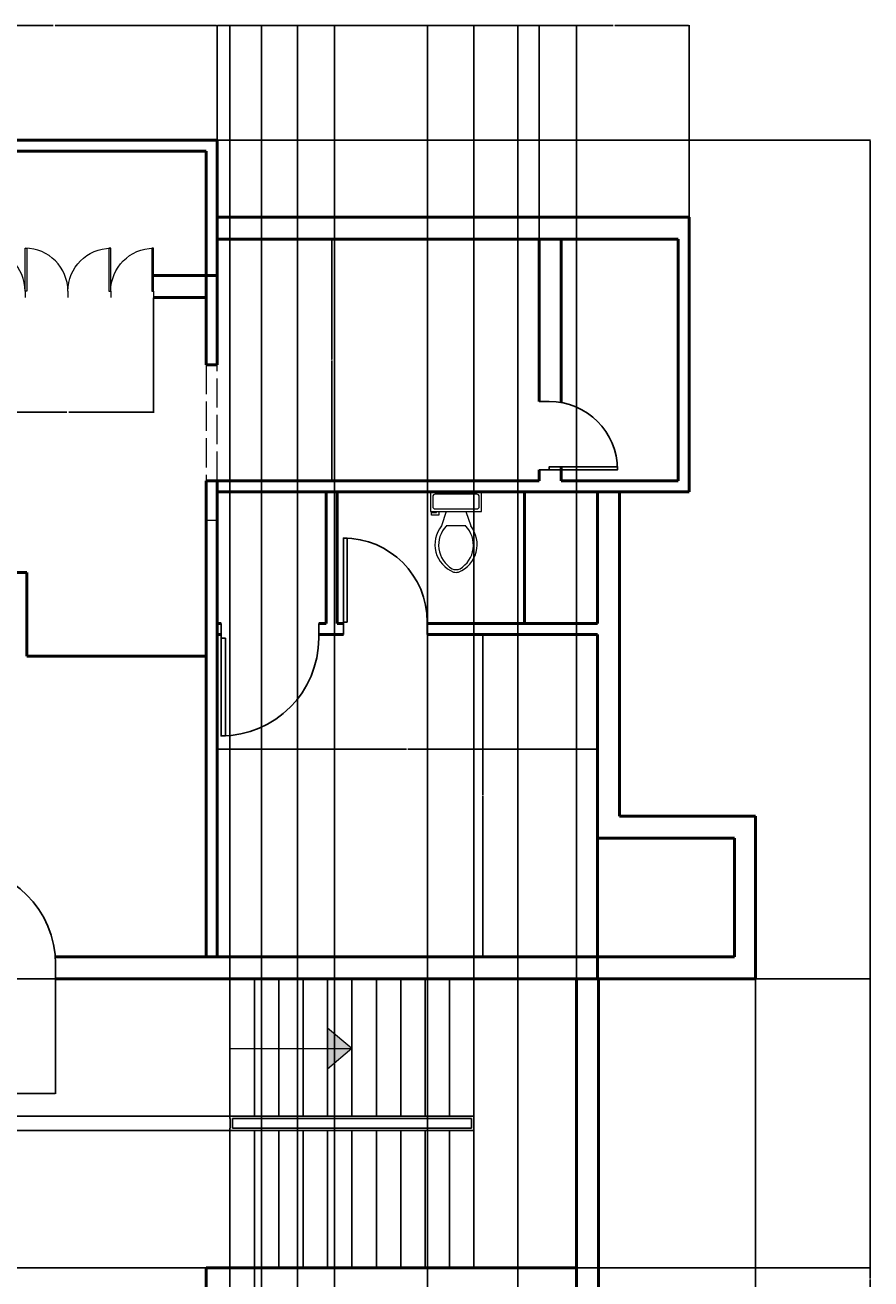
# Model space of a CAD drawing. Units: inches. Extents: x 2032 to 3981, y 840 to 2177.
# Tile 5 of 6: x 2378 to 2725, y 1354 to 1868. Entities that reach past the tile are written whole.
import ezdxf

# ---------------------------------------------------------------- set-up
doc = ezdxf.new("R2010")
doc.units = ezdxf.units.IN
doc.linetypes.add('ACAD_ISO02W100', pattern=[15, 12, -3])
for name, color, linetype, lineweight in [('A-ANNO-DIMS', 2, 'Continuous', 18), ('A-ANNO-SYMB', 2, 'Continuous', 18), ('A-DOOR', 3, 'Continuous', 25), ('A-FLOR-FIXT', 9, 'Continuous', 18), ('A-FLOR-STRS', 7, 'Continuous', 25), ('A-GLAZ', 4, 'Continuous', 18), ('A-WALL', 7, 'Continuous', 50), ('A-WALL-OVHD', 8, 'ACAD_ISO02W100', 18)]:
    doc.layers.add(name, color=color, linetype=linetype, lineweight=lineweight)
doc.styles.get("Standard").update_dxf_attribs({"font": 'arial.ttf'})
doc.dimstyles.get("Standard").update_dxf_attribs({"dimtxt": 0.18, "dimasz": 0.18, "dimexe": 0.18, "dimexo": 0.0625, "dimgap": 0.09, "dimtad": 0, "dimtih": 1, "dimtoh": 1, "dimdec": 4, "dimzin": 0, "dimdsep": 46, "dimtxsty": 'Standard', "dimcen": 0.09, "dimadec": 0, "dimazin": 0, "dimtfac": 1, "dimtdec": 4, "dimtofl": 0, "dimtmove": 0, "dimatfit": 3, "dimfxl": 1, "dimtolj": 1, "dimtzin": 0, "dimarcsym": 0})

# ---------------------------------------------------------------- blocks, each defined once
blk = doc.blocks.new('*U2')
for p, q in [((0, 0), (0, -6)), ((40, 0), (40, -6))]:
    blk.add_line(p, q)
blk.add_lwpolyline([(0, 0), (0, 40), (1.75, 40), (1.75, 0)], close=True)
blk.add_arc((0, 0), 40, 0, 90)
blk = doc.blocks.new('*U4')
for p, q in [((9.5, -6), (9.5, -2)), ((-10, -8.5), (-8, -8.5)), ((-10, -9.5), (-10, -8.5)), ((-7, -9.5), (-10, -9.5)), ((-8, -8.5), (-8, -8)), ((-7, -8), (-7, -9.5)), ((-4, -8), (-6, -14)), ((4, -8), (6, -14)), ((4, -14), (-4, -14))]:
    blk.add_line(p, q)
blk.add_lwpolyline([(10.5, -8), (10.5, 0), (-10.5, 0), (-10.5, -8)], close=True)
for points in [[(-9.5, -2), (-9.5, -6)], [(8.5, -1), (-8.5, -1)], [(-8.5, -7), (8.5, -7)]]:
    blk.add_lwpolyline(points)
for centre, radius, start, end in [((-8.62, -1.88), 0.884, 81.8699, 188.1301), ((8.62, -1.88), 0.884, 351.8699, 98.1301), ((-8.62, -6.12), 0.884, 171.8699, 278.1301), ((8.62, -6.12), 0.884, 261.8699, 8.1301), ((3.52, -21.58), 12.17, 141.4691, 247.9714), ((4.2, -21.82), 11.33, 136.3677, 238.9468), ((-3.52, -21.58), 12.17, 292.0284, 38.5307), ((-4.2, -21.82), 11.33, 301.053, 43.6321), ((0, -27.88), 4, 245.7318, 294.2682), ((0, -29), 4, 254.8605, 285.1395)]:
    blk.add_arc(centre, radius, start, end)
blk = doc.blocks.new('*D14')
at = {"layer": 'A-ANNO-DIMS', "color": 0, "lineweight": -2, "transparency": 16777216}
for p, q in [((2078.89, 1518.9), (2078.89, 840.08)), ((2677.35, 1476.9), (2677.35, 840.08)), ((2079.07, 840.26), (2377.73, 840.26)), ((2677.17, 840.26), (2378.52, 840.26))]:
    blk.add_line(p, q, dxfattribs=at)
at = {"layer": 'A-ANNO-DIMS', "color": 0, "lineweight": 100, "transparency": 16777216}
for points in [[(2079.07, 840.29), (2079.07, 840.23), (2078.89, 840.26)], [(2677.17, 840.29), (2677.17, 840.23), (2677.35, 840.26)]]:
    blk.add_solid(points, dxfattribs=at)
at = {"layer": 'Defpoints', "color": 0, "lineweight": 100, "transparency": 16777216}
for p in [(2078.89, 1518.96), (2677.35, 1476.96), (2677.35, 840.26)]:
    blk.add_point(p, dxfattribs=at)
at = {"layer": 'A-ANNO-DIMS', "color": 0, "transparency": 16777216, "insert": (2378.12, 840.26), "char_height": 0.18, "attachment_point": 5}
blk.add_mtext('\\A1;598.5', dxfattribs=at)
blk = doc.blocks.new('*D15')
at = {"layer": 'A-ANNO-DIMS', "color": 0, "lineweight": -2, "transparency": 16777216}
for p, q in [((2456.69, 1820.52), (2724.53, 1820.52)), ((2724.35, 1820.34), (2724.35, 1354.07)), ((2724.35, 887.44), (2724.35, 1353.71)), ((2476.27, 887.26), (2724.53, 887.26))]:
    blk.add_line(p, q, dxfattribs=at)
at = {"layer": 'A-ANNO-DIMS', "color": 0, "lineweight": 100, "transparency": 16777216}
for points in [[(2724.32, 1820.34), (2724.38, 1820.34), (2724.35, 1820.52)], [(2724.32, 887.44), (2724.38, 887.44), (2724.35, 887.26)]]:
    blk.add_solid(points, dxfattribs=at)
at = {"layer": 'Defpoints', "color": 0, "lineweight": 100, "transparency": 16777216}
for p in [(2456.63, 1820.52), (2476.21, 887.26), (2724.35, 887.26)]:
    blk.add_point(p, dxfattribs=at)
at = {"layer": 'A-ANNO-DIMS', "color": 0, "transparency": 16777216, "insert": (2724.35, 1353.89), "char_height": 0.18, "attachment_point": 5}
blk.add_mtext('\\A1;933.3', dxfattribs=at)
blk = doc.blocks.new('*D19')
at = {"layer": 'A-ANNO-DIMS', "color": 0, "lineweight": -2, "transparency": 16777216}
for p, q in [((2323.13, 1820.58), (2323.13, 1867.7)), ((2323.31, 1867.52), (2389.49, 1867.52)), ((2456.45, 1867.52), (2390.26, 1867.52)), ((2456.63, 1820.58), (2456.63, 1867.7))]:
    blk.add_line(p, q, dxfattribs=at)
at = {"layer": 'A-ANNO-DIMS', "color": 0, "lineweight": 100, "transparency": 16777216}
for points in [[(2323.31, 1867.55), (2323.31, 1867.49), (2323.13, 1867.52)], [(2456.45, 1867.55), (2456.45, 1867.49), (2456.63, 1867.52)]]:
    blk.add_solid(points, dxfattribs=at)
at = {"layer": 'Defpoints', "color": 0, "lineweight": 100, "transparency": 16777216}
for p in [(2456.63, 1867.52), (2323.13, 1820.52), (2456.63, 1820.52)]:
    blk.add_point(p, dxfattribs=at)
at = {"layer": 'A-ANNO-DIMS', "color": 0, "transparency": 16777216, "insert": (2389.88, 1867.52), "char_height": 0.18, "attachment_point": 5}
blk.add_mtext('\\A1;133.5', dxfattribs=at)
blk = doc.blocks.new('*D20')
at = {"layer": 'A-ANNO-DIMS', "color": 0, "lineweight": -2, "transparency": 16777216}
for p, q in [((2456.63, 1820.58), (2456.63, 1867.7)), ((2456.81, 1867.52), (2522.35, 1867.52)), ((2588.45, 1867.52), (2522.91, 1867.52)), ((2588.63, 1780.02), (2588.63, 1867.7))]:
    blk.add_line(p, q, dxfattribs=at)
at = {"layer": 'A-ANNO-DIMS', "color": 0, "lineweight": 100, "transparency": 16777216}
for points in [[(2456.81, 1867.55), (2456.81, 1867.49), (2456.63, 1867.52)], [(2588.45, 1867.55), (2588.45, 1867.49), (2588.63, 1867.52)]]:
    blk.add_solid(points, dxfattribs=at)
at = {"layer": 'Defpoints', "color": 0, "lineweight": 100, "transparency": 16777216}
for p in [(2588.63, 1867.52), (2456.63, 1820.52), (2588.63, 1779.96)]:
    blk.add_point(p, dxfattribs=at)
at = {"layer": 'A-ANNO-DIMS', "color": 0, "transparency": 16777216, "insert": (2522.63, 1867.52), "char_height": 0.18, "attachment_point": 5}
blk.add_mtext('\\A1;132', dxfattribs=at)
blk = doc.blocks.new('*D21')
at = {"layer": 'A-ANNO-DIMS', "color": 0, "lineweight": -2, "transparency": 16777216}
for p, q in [((2588.63, 1780.02), (2588.63, 1867.7)), ((2588.81, 1867.52), (2619.05, 1867.52)), ((2649.95, 1867.52), (2619.7, 1867.52)), ((2650.13, 1789.02), (2650.13, 1867.7))]:
    blk.add_line(p, q, dxfattribs=at)
at = {"layer": 'A-ANNO-DIMS', "color": 0, "lineweight": 100, "transparency": 16777216}
for points in [[(2588.81, 1867.55), (2588.81, 1867.49), (2588.63, 1867.52)], [(2649.95, 1867.55), (2649.95, 1867.49), (2650.13, 1867.52)]]:
    blk.add_solid(points, dxfattribs=at)
at = {"layer": 'Defpoints', "color": 0, "lineweight": 100, "transparency": 16777216}
for p in [(2650.13, 1867.52), (2650.13, 1788.96), (2588.63, 1779.96)]:
    blk.add_point(p, dxfattribs=at)
at = {"layer": 'A-ANNO-DIMS', "color": 0, "transparency": 16777216, "insert": (2619.38, 1867.52), "char_height": 0.18, "attachment_point": 5}
blk.add_mtext('\\A1;61.5', dxfattribs=at)
blk = doc.blocks.new('*D31')
at = {"layer": 'A-ANNO-DIMS', "color": 0, "lineweight": -2, "transparency": 16777216}
for p, q in [((2456.69, 1779.96), (2503.81, 1779.96)), ((2503.63, 1779.78), (2503.63, 1730.64)), ((2503.63, 1681.14), (2503.63, 1730.28)), ((2456.69, 1680.96), (2503.81, 1680.96))]:
    blk.add_line(p, q, dxfattribs=at)
at = {"layer": 'A-ANNO-DIMS', "color": 0, "lineweight": 100, "transparency": 16777216}
for points in [[(2503.6, 1779.78), (2503.66, 1779.78), (2503.63, 1779.96)], [(2503.6, 1681.14), (2503.66, 1681.14), (2503.63, 1680.96)]]:
    blk.add_solid(points, dxfattribs=at)
at = {"layer": 'Defpoints', "color": 0, "lineweight": 100, "transparency": 16777216}
for p in [(2456.63, 1779.96), (2456.63, 1680.96), (2503.63, 1680.96)]:
    blk.add_point(p, dxfattribs=at)
at = {"layer": 'A-ANNO-DIMS', "color": 0, "transparency": 16777216, "insert": (2503.63, 1730.46), "char_height": 0.18, "attachment_point": 5}
blk.add_mtext('\\A1;99', dxfattribs=at)
blk = doc.blocks.new('*D32')
at = {"layer": 'A-ANNO-DIMS', "color": 0, "lineweight": -2, "transparency": 16777216}
for p, q in [((2360.39, 1756), (2360.39, 1708.89)), ((2430.64, 1756), (2430.64, 1708.89)), ((2360.57, 1709.07), (2395.12, 1709.07)), ((2430.46, 1709.07), (2395.91, 1709.07))]:
    blk.add_line(p, q, dxfattribs=at)
at = {"layer": 'A-ANNO-DIMS', "color": 0, "lineweight": 100, "transparency": 16777216}
for points in [[(2360.57, 1709.1), (2360.57, 1709.04), (2360.39, 1709.07)], [(2430.46, 1709.1), (2430.46, 1709.04), (2430.64, 1709.07)]]:
    blk.add_solid(points, dxfattribs=at)
at = {"layer": 'Defpoints', "color": 0, "lineweight": 100, "transparency": 16777216}
for p in [(2360.39, 1756.07), (2430.64, 1756.07), (2360.39, 1709.07)]:
    blk.add_point(p, dxfattribs=at)
at = {"layer": 'A-ANNO-DIMS', "color": 0, "transparency": 16777216, "insert": (2395.51, 1709.07), "char_height": 0.18, "attachment_point": 5}
blk.add_mtext('\\A1;70.24', dxfattribs=at)
blk = doc.blocks.new('*D35')
at = {"layer": 'A-ANNO-DIMS', "color": 0, "lineweight": -2, "transparency": 16777216}
for p, q in [((2456.63, 1617.9), (2456.63, 1570.78)), ((2612.63, 1617.9), (2612.63, 1570.78)), ((2456.81, 1570.96), (2534.35, 1570.96)), ((2612.45, 1570.96), (2534.91, 1570.96))]:
    blk.add_line(p, q, dxfattribs=at)
at = {"layer": 'A-ANNO-DIMS', "color": 0, "lineweight": 100, "transparency": 16777216}
for points in [[(2456.81, 1570.99), (2456.81, 1570.93), (2456.63, 1570.96)], [(2612.45, 1570.99), (2612.45, 1570.93), (2612.63, 1570.96)]]:
    blk.add_solid(points, dxfattribs=at)
at = {"layer": 'Defpoints', "color": 0, "lineweight": 100, "transparency": 16777216}
for p in [(2456.63, 1617.96), (2612.63, 1617.96), (2456.63, 1570.96)]:
    blk.add_point(p, dxfattribs=at)
at = {"layer": 'A-ANNO-DIMS', "color": 0, "transparency": 16777216, "insert": (2534.63, 1570.96), "char_height": 0.18, "attachment_point": 5}
blk.add_mtext('\\A1;156', dxfattribs=at)
blk = doc.blocks.new('*D36')
at = {"layer": 'A-ANNO-DIMS', "color": 0, "lineweight": -2, "transparency": 16777216}
for p, q in [((2612.57, 1617.96), (2565.45, 1617.96)), ((2565.63, 1617.78), (2565.63, 1552.14)), ((2565.63, 1486.14), (2565.63, 1551.78)), ((2612.57, 1485.96), (2565.45, 1485.96))]:
    blk.add_line(p, q, dxfattribs=at)
at = {"layer": 'A-ANNO-DIMS', "color": 0, "lineweight": 100, "transparency": 16777216}
for points in [[(2565.6, 1617.78), (2565.66, 1617.78), (2565.63, 1617.96)], [(2565.6, 1486.14), (2565.66, 1486.14), (2565.63, 1485.96)]]:
    blk.add_solid(points, dxfattribs=at)
at = {"layer": 'Defpoints', "color": 0, "lineweight": 100, "transparency": 16777216}
for p in [(2565.63, 1617.96), (2612.63, 1617.96), (2612.63, 1485.96)]:
    blk.add_point(p, dxfattribs=at)
at = {"layer": 'A-ANNO-DIMS', "color": 0, "transparency": 16777216, "insert": (2565.63, 1551.96), "char_height": 0.18, "attachment_point": 5}
blk.add_mtext('\\A1;132', dxfattribs=at)
blk = doc.blocks.new('*D37')
at = {"layer": 'A-ANNO-DIMS', "color": 0, "lineweight": -2, "transparency": 16777216}
for p, q in [((2350.44, 1476.9), (2350.44, 1429.78)), ((2390.44, 1476.9), (2390.44, 1429.78)), ((2350.62, 1429.96), (2370.22, 1429.96)), ((2390.26, 1429.96), (2370.66, 1429.96))]:
    blk.add_line(p, q, dxfattribs=at)
at = {"layer": 'A-ANNO-DIMS', "color": 0, "lineweight": 100, "transparency": 16777216}
for points in [[(2350.62, 1429.99), (2350.62, 1429.93), (2350.44, 1429.96)], [(2390.26, 1429.99), (2390.26, 1429.93), (2390.44, 1429.96)]]:
    blk.add_solid(points, dxfattribs=at)
at = {"layer": 'Defpoints', "color": 0, "lineweight": 100, "transparency": 16777216}
for p in [(2350.44, 1476.96), (2390.44, 1476.96), (2350.44, 1429.96)]:
    blk.add_point(p, dxfattribs=at)
at = {"layer": 'A-ANNO-DIMS', "color": 0, "transparency": 16777216, "insert": (2370.44, 1429.96), "char_height": 0.18, "attachment_point": 5}
blk.add_mtext('\\A1;40', dxfattribs=at)
blk = doc.blocks.new('*D51')
at = {"layer": 'A-ANNO-DIMS', "color": 0, "lineweight": -2, "transparency": 16777216}
for p, q in [((2474.93, 1231.02), (2474.93, 1867.7)), ((2475.11, 1867.52), (2481.81, 1867.52)), ((2489.42, 1867.52), (2482.72, 1867.52)), ((2489.6, 1231.02), (2489.6, 1867.7))]:
    blk.add_line(p, q, dxfattribs=at)
at = {"layer": 'A-ANNO-DIMS', "color": 0, "lineweight": 100, "transparency": 16777216}
for points in [[(2475.11, 1867.55), (2475.11, 1867.49), (2474.93, 1867.52)], [(2489.42, 1867.55), (2489.42, 1867.49), (2489.6, 1867.52)]]:
    blk.add_solid(points, dxfattribs=at)
at = {"layer": 'Defpoints', "color": 0, "lineweight": 100, "transparency": 16777216}
for p in [(2489.6, 1867.52), (2474.93, 1230.96), (2489.6, 1230.96)]:
    blk.add_point(p, dxfattribs=at)
at = {"layer": 'A-ANNO-DIMS', "color": 0, "transparency": 16777216, "insert": (2482.27, 1867.52), "char_height": 0.18, "attachment_point": 5}
blk.add_mtext('\\A1;14.668', dxfattribs=at)
blk = doc.blocks.new('*D52')
at = {"layer": 'A-ANNO-DIMS', "color": 0, "lineweight": -2, "transparency": 16777216}
for p, q in [((2489.6, 1231.02), (2489.6, 1867.7)), ((2489.78, 1867.52), (2496.71, 1867.52)), ((2504.55, 1867.52), (2497.62, 1867.52)), ((2504.73, 1228.5), (2504.73, 1867.7))]:
    blk.add_line(p, q, dxfattribs=at)
at = {"layer": 'A-ANNO-DIMS', "color": 0, "lineweight": 100, "transparency": 16777216}
for points in [[(2489.78, 1867.55), (2489.78, 1867.49), (2489.6, 1867.52)], [(2504.55, 1867.55), (2504.55, 1867.49), (2504.73, 1867.52)]]:
    blk.add_solid(points, dxfattribs=at)
at = {"layer": 'Defpoints', "color": 0, "lineweight": 100, "transparency": 16777216}
for p in [(2504.73, 1867.52), (2489.6, 1230.96), (2504.73, 1228.44)]:
    blk.add_point(p, dxfattribs=at)
at = {"layer": 'A-ANNO-DIMS', "color": 0, "transparency": 16777216, "insert": (2497.17, 1867.52), "char_height": 0.18, "attachment_point": 5}
blk.add_mtext('\\A1;15.127', dxfattribs=at)
blk = doc.blocks.new('*D53')
at = {"layer": 'A-ANNO-DIMS', "color": 0, "lineweight": -2, "transparency": 16777216}
for p, q in [((2504.73, 1228.5), (2504.73, 1867.7)), ((2504.91, 1867.52), (2523.42, 1867.52)), ((2542.71, 1867.52), (2524.2, 1867.52)), ((2542.89, 1228.5), (2542.89, 1867.7))]:
    blk.add_line(p, q, dxfattribs=at)
at = {"layer": 'A-ANNO-DIMS', "color": 0, "lineweight": 100, "transparency": 16777216}
for points in [[(2504.91, 1867.55), (2504.91, 1867.49), (2504.73, 1867.52)], [(2542.71, 1867.55), (2542.71, 1867.49), (2542.89, 1867.52)]]:
    blk.add_solid(points, dxfattribs=at)
at = {"layer": 'Defpoints', "color": 0, "lineweight": 100, "transparency": 16777216}
for p in [(2542.89, 1867.52), (2504.73, 1228.44), (2542.89, 1228.44)]:
    blk.add_point(p, dxfattribs=at)
at = {"layer": 'A-ANNO-DIMS', "color": 0, "transparency": 16777216, "insert": (2523.81, 1867.52), "char_height": 0.18, "attachment_point": 5}
blk.add_mtext('\\A1;38.16', dxfattribs=at)
blk = doc.blocks.new('*D54')
at = {"layer": 'A-ANNO-DIMS', "color": 0, "lineweight": -2, "transparency": 16777216}
for p, q in [((2542.89, 1228.5), (2542.89, 1867.7)), ((2543.07, 1867.52), (2560.95, 1867.52)), ((2579.75, 1867.52), (2561.88, 1867.52)), ((2579.93, 1207.02), (2579.93, 1867.7))]:
    blk.add_line(p, q, dxfattribs=at)
at = {"layer": 'A-ANNO-DIMS', "color": 0, "lineweight": 100, "transparency": 16777216}
for points in [[(2543.07, 1867.55), (2543.07, 1867.49), (2542.89, 1867.52)], [(2579.75, 1867.55), (2579.75, 1867.49), (2579.93, 1867.52)]]:
    blk.add_solid(points, dxfattribs=at)
at = {"layer": 'Defpoints', "color": 0, "lineweight": 100, "transparency": 16777216}
for p in [(2579.93, 1867.52), (2542.89, 1228.44), (2579.93, 1206.96)]:
    blk.add_point(p, dxfattribs=at)
at = {"layer": 'A-ANNO-DIMS', "color": 0, "transparency": 16777216, "insert": (2561.41, 1867.52), "char_height": 0.18, "attachment_point": 5}
blk.add_mtext('\\A1;37.045', dxfattribs=at)
blk = doc.blocks.new('*D55')
at = {"layer": 'A-ANNO-DIMS', "color": 0, "lineweight": -2, "transparency": 16777216}
for p, q in [((2579.93, 1207.02), (2579.93, 1867.7)), ((2580.11, 1867.52), (2591.71, 1867.52)), ((2603.75, 1867.52), (2592.15, 1867.52)), ((2603.93, 1231.02), (2603.93, 1867.7))]:
    blk.add_line(p, q, dxfattribs=at)
at = {"layer": 'A-ANNO-DIMS', "color": 0, "lineweight": 100, "transparency": 16777216}
for points in [[(2580.11, 1867.55), (2580.11, 1867.49), (2579.93, 1867.52)], [(2603.75, 1867.55), (2603.75, 1867.49), (2603.93, 1867.52)]]:
    blk.add_solid(points, dxfattribs=at)
at = {"layer": 'Defpoints', "color": 0, "lineweight": 100, "transparency": 16777216}
for p in [(2603.93, 1867.52), (2603.93, 1230.96), (2579.93, 1206.96)]:
    blk.add_point(p, dxfattribs=at)
at = {"layer": 'A-ANNO-DIMS', "color": 0, "transparency": 16777216, "insert": (2591.93, 1867.52), "char_height": 0.18, "attachment_point": 5}
blk.add_mtext('\\A1;24', dxfattribs=at)
blk = doc.blocks.new('*D63')
at = {"layer": 'A-ANNO-DIMS', "color": 0, "lineweight": -2, "transparency": 16777216}
for p, q in [((2461.93, 1477.02), (2461.93, 1867.7)), ((2462.11, 1867.52), (2511.65, 1867.52)), ((2561.75, 1867.52), (2512.21, 1867.52)), ((2561.93, 1477.02), (2561.93, 1867.7))]:
    blk.add_line(p, q, dxfattribs=at)
at = {"layer": 'A-ANNO-DIMS', "color": 0, "lineweight": 100, "transparency": 16777216}
for points in [[(2462.11, 1867.55), (2462.11, 1867.49), (2461.93, 1867.52)], [(2561.75, 1867.55), (2561.75, 1867.49), (2561.93, 1867.52)]]:
    blk.add_solid(points, dxfattribs=at)
at = {"layer": 'Defpoints', "color": 0, "lineweight": 100, "transparency": 16777216}
for p in [(2561.93, 1867.52), (2461.93, 1476.96), (2561.93, 1476.96)]:
    blk.add_point(p, dxfattribs=at)
at = {"layer": 'A-ANNO-DIMS', "color": 0, "transparency": 16777216, "insert": (2511.93, 1867.52), "char_height": 0.18, "attachment_point": 5}
blk.add_mtext('\\A1;100', dxfattribs=at)
blk = doc.blocks.new('*D64')
at = {"layer": 'A-ANNO-DIMS', "color": 0, "lineweight": -2, "transparency": 16777216}
for p, q in [((2561.93, 1477.02), (2561.93, 1867.7)), ((2562.11, 1867.52), (2582.71, 1867.52)), ((2603.75, 1867.52), (2583.16, 1867.52)), ((2603.93, 1477.02), (2603.93, 1867.7))]:
    blk.add_line(p, q, dxfattribs=at)
at = {"layer": 'A-ANNO-DIMS', "color": 0, "lineweight": 100, "transparency": 16777216}
for points in [[(2562.11, 1867.55), (2562.11, 1867.49), (2561.93, 1867.52)], [(2603.75, 1867.55), (2603.75, 1867.49), (2603.93, 1867.52)]]:
    blk.add_solid(points, dxfattribs=at)
at = {"layer": 'Defpoints', "color": 0, "lineweight": 100, "transparency": 16777216}
for p in [(2603.93, 1867.52), (2561.93, 1476.96), (2603.93, 1476.96)]:
    blk.add_point(p, dxfattribs=at)
at = {"layer": 'A-ANNO-DIMS', "color": 0, "transparency": 16777216, "insert": (2582.93, 1867.52), "char_height": 0.18, "attachment_point": 5}
blk.add_mtext('\\A1;42', dxfattribs=at)
blk = doc.blocks.new('*D65')
at = {"layer": 'A-ANNO-DIMS', "color": 0, "lineweight": -2, "transparency": 16777216}
for p, q in [((2461.93, 1358.4), (2461.93, 840.08)), ((2471.93, 1358.4), (2471.93, 840.08)), ((2462.11, 840.26), (2466.72, 840.26)), ((2471.75, 840.26), (2467.14, 840.26))]:
    blk.add_line(p, q, dxfattribs=at)
at = {"layer": 'A-ANNO-DIMS', "color": 0, "lineweight": 100, "transparency": 16777216}
for points in [[(2462.11, 840.29), (2462.11, 840.23), (2461.93, 840.26)], [(2471.75, 840.29), (2471.75, 840.23), (2471.93, 840.26)]]:
    blk.add_solid(points, dxfattribs=at)
at = {"layer": 'Defpoints', "color": 0, "lineweight": 100, "transparency": 16777216}
for p in [(2461.93, 1358.46), (2471.93, 1358.46), (2471.93, 840.26)]:
    blk.add_point(p, dxfattribs=at)
at = {"layer": 'A-ANNO-DIMS', "color": 0, "transparency": 16777216, "insert": (2466.93, 840.26), "char_height": 0.18, "attachment_point": 5}
blk.add_mtext('\\A1;10', dxfattribs=at)
blk = doc.blocks.new('*D66')
at = {"layer": 'A-ANNO-DIMS', "color": 0, "lineweight": -2, "transparency": 16777216}
for p, q in [((2461.87, 1414.71), (2031.71, 1414.71)), ((2031.89, 1414.53), (2031.89, 1386.77)), ((2031.89, 1358.64), (2031.89, 1386.4)), ((2461.87, 1358.46), (2031.71, 1358.46))]:
    blk.add_line(p, q, dxfattribs=at)
at = {"layer": 'A-ANNO-DIMS', "color": 0, "lineweight": 100, "transparency": 16777216}
for points in [[(2031.86, 1414.53), (2031.92, 1414.53), (2031.89, 1414.71)], [(2031.86, 1358.64), (2031.92, 1358.64), (2031.89, 1358.46)]]:
    blk.add_solid(points, dxfattribs=at)
at = {"layer": 'Defpoints', "color": 0, "lineweight": 100, "transparency": 16777216}
for p in [(2461.93, 1414.71), (2031.89, 1358.46), (2461.93, 1358.46)]:
    blk.add_point(p, dxfattribs=at)
at = {"layer": 'A-ANNO-DIMS', "color": 0, "transparency": 16777216, "insert": (2031.89, 1386.58), "char_height": 0.18, "attachment_point": 5}
blk.add_mtext('\\A1;56.25', dxfattribs=at)
blk = doc.blocks.new('*D67')
at = {"layer": 'A-ANNO-DIMS', "color": 0, "lineweight": -2, "transparency": 16777216}
for p, q in [((2461.87, 1476.96), (2031.71, 1476.96)), ((2031.89, 1476.78), (2031.89, 1449.02)), ((2031.89, 1420.89), (2031.89, 1448.65)), ((2461.87, 1420.71), (2031.71, 1420.71))]:
    blk.add_line(p, q, dxfattribs=at)
at = {"layer": 'A-ANNO-DIMS', "color": 0, "lineweight": 100, "transparency": 16777216}
for points in [[(2031.86, 1476.78), (2031.92, 1476.78), (2031.89, 1476.96)], [(2031.86, 1420.89), (2031.92, 1420.89), (2031.89, 1420.71)]]:
    blk.add_solid(points, dxfattribs=at)
at = {"layer": 'Defpoints', "color": 0, "lineweight": 100, "transparency": 16777216}
for p in [(2461.93, 1476.96), (2031.89, 1420.71), (2461.93, 1420.71)]:
    blk.add_point(p, dxfattribs=at)
at = {"layer": 'A-ANNO-DIMS', "color": 0, "transparency": 16777216, "insert": (2031.89, 1448.83), "char_height": 0.18, "attachment_point": 5}
blk.add_mtext('\\A1;56.25', dxfattribs=at)
blk = doc.blocks.new('*D68')
at = {"layer": 'A-ANNO-DIMS', "color": 0, "lineweight": -2, "transparency": 16777216}
for p, q in [((2604, 1476.96), (2724.53, 1476.96)), ((2724.35, 1476.78), (2724.35, 1417.89)), ((2724.35, 1358.64), (2724.35, 1417.53)), ((2604, 1358.46), (2724.53, 1358.46))]:
    blk.add_line(p, q, dxfattribs=at)
at = {"layer": 'A-ANNO-DIMS', "color": 0, "lineweight": 100, "transparency": 16777216}
for points in [[(2724.32, 1476.78), (2724.38, 1476.78), (2724.35, 1476.96)], [(2724.32, 1358.64), (2724.38, 1358.64), (2724.35, 1358.46)]]:
    blk.add_solid(points, dxfattribs=at)
at = {"layer": 'Defpoints', "color": 0, "lineweight": 100, "transparency": 16777216}
for p in [(2603.93, 1476.96), (2724.35, 1476.96), (2603.93, 1358.46)]:
    blk.add_point(p, dxfattribs=at)
at = {"layer": 'A-ANNO-DIMS', "color": 0, "transparency": 16777216, "insert": (2724.35, 1417.71), "char_height": 0.18, "attachment_point": 5}
blk.add_mtext('\\A1;118.5', dxfattribs=at)

msp = doc.modelspace()

# ---------------------------------------------------------------- hatches: boundary and pattern name
at = {"layer": 'A-ANNO-SYMB'}
h = msp.add_hatch(color=256, dxfattribs=at)
h.dxf.hatch_style = 1
h.paths.add_polyline_path([(2511.9346, 1448.3334), (2501.9346, 1448.3334), (2501.9346, 1439.9572)])
h.paths.add_polyline_path([(2501.9346, 1456.7096), (2501.9346, 1448.3334), (2511.9346, 1448.3334)])

# ---------------------------------------------------------------- linework, layer by layer
for p, q in [((2511.9346, 1448.3334), (2501.9346, 1456.7096)), ((2461.9346, 1448.3334), (2511.9346, 1448.3334)), ((2511.9346, 1448.3334), (2501.9346, 1439.9572))]:
    msp.add_line(p, q, dxfattribs=at)
at = {"layer": 'A-FLOR-STRS'}
for p, q in [((2461.9346, 1419.7084), (2461.9346, 1476.9584)), ((2471.9346, 1420.7084), (2471.9346, 1476.9584)), ((2481.9346, 1420.7084), (2481.9346, 1476.9584)), ((2491.9346, 1420.7084), (2491.9346, 1476.9584)), ((2501.9346, 1420.7084), (2501.9346, 1476.9584)), ((2511.9346, 1420.7084), (2511.9346, 1476.9584)), ((2521.9346, 1420.7084), (2521.9346, 1476.9584)), ((2531.9346, 1420.7084), (2531.9346, 1476.9584)), ((2541.9346, 1420.7084), (2541.9346, 1476.9584)), ((2551.9346, 1420.7084), (2551.9346, 1476.9584)), ((2561.9346, 1358.4584), (2561.9346, 1476.9584)), ((2561.9346, 1420.7084), (2461.9346, 1420.7084)), ((2461.9519, 1419.7084), (2461.9346, 1419.7084)), ((2461.9519, 1415.7084), (2461.9519, 1419.7084)), ((2560.9346, 1419.7084), (2462.9434, 1419.7084)), ((2462.9434, 1415.7084), (2462.9434, 1419.7084)), ((2560.9346, 1415.7084), (2560.9346, 1419.7084)), ((2461.9346, 1358.4584), (2461.9346, 1415.7084)), ((2461.9519, 1415.7084), (2461.9346, 1415.7084)), ((2561.9346, 1414.7084), (2461.9346, 1414.7084)), ((2560.9346, 1415.7084), (2462.9434, 1415.7084)), ((2471.9346, 1358.4584), (2471.9346, 1414.7084)), ((2481.9346, 1358.4584), (2481.9346, 1414.7084)), ((2491.9346, 1358.4584), (2491.9346, 1414.7084)), ((2501.9346, 1358.4584), (2501.9346, 1414.7084)), ((2511.9346, 1358.4584), (2511.9346, 1414.7084)), ((2521.9346, 1358.4584), (2521.9346, 1414.7084)), ((2531.9346, 1358.4584), (2531.9346, 1414.7084)), ((2541.9346, 1358.4584), (2541.9346, 1414.7084)), ((2551.9346, 1358.4584), (2551.9346, 1414.7084)), ((2603.9346, 1358.4584), (2561.9346, 1358.4584))]:
    msp.add_line(p, q, dxfattribs=at)
at = {"layer": 'A-WALL'}
for p, q in [((2323.1278, 1820.5217), (2456.6278, 1820.5217)), ((2456.6278, 1788.9584), (2456.6278, 1820.5217)), ((2327.6278, 1816.0217), (2452.1278, 1816.0217)), ((2452.1278, 1816.0217), (2452.1278, 1756.0659)), ((2456.6278, 1788.9584), (2456.6278, 1765.0659)), ((2456.6278, 1788.9584), (2597.6278, 1788.9584)), ((2597.6278, 1788.9584), (2650.1278, 1788.9584)), ((2650.1278, 1788.9584), (2650.1278, 1676.4584)), ((2456.6278, 1779.9584), (2588.6278, 1779.9584)), ((2588.6278, 1779.9584), (2588.6278, 1713.4753)), ((2588.6278, 1779.9584), (2597.6278, 1779.9584)), ((2597.6278, 1779.9584), (2597.6278, 1713.0593)), ((2597.6278, 1779.9584), (2645.6278, 1779.9584)), ((2645.6278, 1779.9584), (2645.6278, 1680.9584)), ((2429.867, 1765.0659), (2456.6278, 1765.0659)), ((2456.6278, 1765.0659), (2456.6278, 1728.454)), ((2430.6353, 1756.0659), (2452.1278, 1756.0659)), ((2452.1278, 1756.0659), (2452.1278, 1728.454)), ((2452.1278, 1728.454), (2456.6278, 1728.454)), ((2588.6278, 1685.5116), (2588.6278, 1680.9584)), ((2597.6278, 1686.735), (2597.6278, 1680.9584)), ((2456.6278, 1680.9584), (2452.1278, 1680.9584)), ((2452.1278, 1680.9584), (2452.1278, 1609.0659)), ((2588.6278, 1680.9584), (2456.6278, 1680.9584)), ((2456.6278, 1680.9584), (2456.6278, 1609.0659)), ((2645.6278, 1680.9584), (2597.6278, 1680.9584)), ((2597.6278, 1676.4584), (2456.6278, 1676.4584)), ((2456.6278, 1676.4584), (2612.6278, 1676.4584)), ((2501.3318, 1622.4584), (2501.3318, 1676.4584)), ((2505.8318, 1622.4584), (2505.8318, 1676.4584)), ((2582.6913, 1676.4584), (2582.6913, 1622.4584)), ((2650.1278, 1676.4584), (2597.6278, 1676.4584)), ((2612.6278, 1676.4584), (2612.6278, 1622.4584)), ((2621.6278, 1676.4584), (2621.6278, 1617.9584)), ((2378.7092, 1643.4584), (2269.1278, 1643.4584)), ((2378.7092, 1609.0659), (2378.7092, 1643.4584)), ((2458.3109, 1622.4584), (2456.6278, 1622.4584)), ((2501.3318, 1622.4584), (2498.3109, 1622.4584)), ((2508.4235, 1622.4584), (2505.8318, 1622.4584)), ((2612.6278, 1622.4584), (2542.8282, 1622.4584)), ((2452.1278, 1617.9584), (2452.1278, 1485.9584)), ((2456.6278, 1617.9584), (2456.6278, 1485.9584)), ((2458.3109, 1617.9584), (2456.6278, 1617.9584)), ((2508.4235, 1617.9584), (2498.3109, 1617.9584)), ((2508.4235, 1617.9584), (2501.3318, 1617.9584)), ((2612.6278, 1617.9584), (2542.8282, 1617.9584)), ((2612.6278, 1617.9584), (2542.8282, 1617.9584)), ((2612.6278, 1617.9584), (2612.6278, 1485.9584)), ((2621.6278, 1617.9584), (2621.6278, 1543.5447)), ((2452.1278, 1609.0659), (2378.7092, 1609.0659)), ((2612.6278, 1476.9584), (2612.6278, 1543.2223)), ((2677.3537, 1543.5447), (2621.6278, 1543.5447)), ((2677.3537, 1476.9584), (2677.3537, 1543.5447)), ((2621.6278, 1534.5447), (2612.6278, 1534.5447)), ((2668.8065, 1534.5447), (2621.6278, 1534.5447)), ((2668.8065, 1485.9584), (2668.8065, 1534.5447)), ((2390.3256, 1485.9584), (2612.6278, 1485.9584)), ((2612.6278, 1485.9584), (2612.6278, 1476.9584)), ((2612.6278, 1485.9584), (2625.0039, 1485.9584)), ((2621.6278, 1485.9584), (2668.8065, 1485.9584)), ((2452.1278, 1476.9584), (2390.4382, 1476.9584)), ((2452.1278, 1476.9584), (2621.6278, 1476.9584)), ((2603.9346, 1239.9584), (2603.9346, 1476.9584)), ((2612.9346, 1230.9584), (2612.9346, 1476.9584)), ((2621.6278, 1476.9584), (2677.3537, 1476.9584)), ((2603.9346, 1358.4584), (2452.1278, 1358.4584)), ((2452.1278, 1349.4584), (2452.1278, 1358.4584))]:
    msp.add_line(p, q, dxfattribs=at)
at = {"layer": 'A-WALL-OVHD'}
msp.add_line((2452.1278, 1664.8434), (2456.6278, 1664.8434), dxfattribs=at)
msp.add_lwpolyline([(2452.1278, 1680.9584), (2456.6278, 1680.9584), (2456.6278, 1728.454), (2452.1278, 1728.454)], close=True, dxfattribs=at)

# ---------------------------------------------------------------- block references
at = {"layer": 'A-DOOR', "xscale": -0.6990928804041083, "yscale": 0.6990928804041083, "zscale": 0.6990928804041083, "rotation": 270}
msp.add_blockref('*U2', (2592.8224, 1685.5116), dxfattribs=at)
at = {"layer": 'A-DOOR', "xscale": 0.8601163335718837, "yscale": 0.8601163335718837, "zscale": 0.8601163335718837}
msp.add_blockref('*U2', (2508.4235, 1623.1191), dxfattribs=at)
at = {"layer": 'A-DOOR', "xscale": -1, "rotation": 180}
msp.add_blockref('*U2', (2458.3109, 1616.4584), dxfattribs=at)
at = {"layer": 'A-DOOR'}
msp.add_blockref('*U2', (2350.4382, 1482.9584), dxfattribs=at)
at = {"layer": 'A-FLOR-FIXT'}
msp.add_blockref('*U4', (2554.6017, 1676.4584), dxfattribs=at)
at = {"layer": 'A-GLAZ', "yscale": 0.4390204122695697, "zscale": 0.4390204122695697}
for p, xscale in [((2360.392, 1758.7001), 0.4390204122695697), ((2377.9528, 1758.7001), 0.4390204122695697), ((2413.0745, 1758.7001), -0.4390204122695697), ((2430.6353, 1758.7001), -0.4390204122695697)]:
    msp.add_blockref('*U2', p, dxfattribs=dict(at, xscale=xscale))

# ---------------------------------------------------------------- dimensions: what is measured, and where the dimension line sits
at = {"layer": 'A-ANNO-DIMS'}
for base, p1, p2, override, picture, middle in [((2456.6278, 1867.5217), (2323.1278, 1820.5217), (2456.6278, 1820.5217), {"dimdec": 1, "dimlfac": 1, "dimrnd": 0, "dimzin": 0, "dimdsep": 46, "dimlunit": 2}, '*D19', (2389.8778, 1867.5217)), ((2588.6278, 1867.5217), (2456.6278, 1820.5217), (2588.6278, 1779.9584), {"dimdec": 0, "dimlfac": 1, "dimrnd": 0, "dimzin": 0, "dimdsep": 46, "dimlunit": 2}, '*D20', (2522.6278, 1867.5217)), ((2561.9346, 1867.5217), (2461.9346, 1476.9584), (2561.9346, 1476.9584), {"dimdec": 0, "dimlfac": 1, "dimrnd": 0, "dimzin": 0, "dimdsep": 46, "dimlunit": 2}, '*D63', (2511.9346, 1867.5217)), ((2489.6025, 1867.5217), (2474.9346, 1230.9584), (2489.6025, 1230.9584), {"dimdec": 3, "dimlfac": 1, "dimrnd": 0, "dimzin": 0, "dimdsep": 46, "dimlunit": 2}, '*D51', (2482.2686, 1867.5217)), ((2504.7296, 1867.5217), (2489.6025, 1230.9584), (2504.7296, 1228.4424), {"dimdec": 3, "dimlfac": 1, "dimrnd": 0, "dimzin": 0, "dimdsep": 46, "dimlunit": 2}, '*D52', (2497.1661, 1867.5217)), ((2542.8893, 1867.5217), (2504.7296, 1228.4424), (2542.8893, 1228.4424), {"dimdec": 2, "dimlfac": 1, "dimrnd": 0, "dimzin": 0, "dimdsep": 46, "dimlunit": 2}, '*D53', (2523.8094, 1867.5217)), ((2579.9346, 1867.5217), (2542.8893, 1228.4424), (2579.9346, 1206.9584), {"dimdec": 3, "dimlfac": 1, "dimrnd": 0, "dimzin": 0, "dimdsep": 46, "dimlunit": 2}, '*D54', (2561.412, 1867.5217)), ((2603.9346, 1867.5217), (2561.9346, 1476.9584), (2603.9346, 1476.9584), {"dimdec": 0, "dimlfac": 1, "dimrnd": 0, "dimzin": 0, "dimdsep": 46, "dimlunit": 2}, '*D64', (2582.9346, 1867.5217)), ((2603.9346, 1867.5217), (2579.9346, 1206.9584), (2603.9346, 1230.9584), {"dimdec": 0, "dimlfac": 1, "dimrnd": 0, "dimzin": 0, "dimdsep": 46, "dimlunit": 2}, '*D55', (2591.9346, 1867.5217)), ((2650.1278, 1867.5217), (2588.6278, 1779.9584), (2650.1278, 1788.9584), {"dimdec": 1, "dimlfac": 1, "dimrnd": 0, "dimzin": 0, "dimdsep": 46, "dimlunit": 2}, '*D21', (2619.3778, 1867.5217)), ((2677.3537, 840.2551), (2078.8911, 1518.9584), (2677.3537, 1476.9584), {"dimdec": 1, "dimlfac": 1, "dimrnd": 0, "dimzin": 0, "dimdsep": 46, "dimlunit": 2}, '*D14', (2378.1224, 840.2551)), ((2471.9346, 840.2551), (2461.9346, 1358.4584), (2471.9346, 1358.4584), {"dimdec": 0, "dimlfac": 1, "dimrnd": 0, "dimzin": 0, "dimdsep": 46, "dimlunit": 2}, '*D65', (2466.9346, 840.2551))]:
    dim = msp.add_linear_dim(base=base, p1=p1, p2=p2, dimstyle='Standard', override=override, dxfattribs=at)
    dim.commit()
    dim.dimension.update_dxf_attribs({"geometry": picture, "text_midpoint": middle})
for base, p1, p2, angle, override, picture, middle in [((2724.3537, 887.2551), (2456.6278, 1820.5217), (2476.2092, 887.2551), 90, {"dimdec": 1, "dimlfac": 1, "dimrnd": 0, "dimzin": 0, "dimdsep": 46, "dimlunit": 2}, '*D15', (2724.3537, 1353.8884)), ((2503.6278, 1680.9584), (2456.6278, 1779.9584), (2456.6278, 1680.9584), 270, {"dimdec": 0, "dimlfac": 1, "dimrnd": 0, "dimzin": 0, "dimdsep": 46, "dimlunit": 2}, '*D31', (2503.6278, 1730.4584)), ((2360.392, 1709.0659), (2430.6353, 1756.0659), (2360.392, 1756.0659), 180, {"dimdec": 2, "dimlfac": 1, "dimrnd": 0, "dimzin": 0, "dimdsep": 46, "dimlunit": 2}, '*D32', (2395.5137, 1709.0659)), ((2456.6278, 1570.9584), (2612.6278, 1617.9584), (2456.6278, 1617.9584), 180, {"dimdec": 0, "dimlfac": 1, "dimrnd": 0, "dimzin": 0, "dimdsep": 46, "dimlunit": 2}, '*D35', (2534.6278, 1570.9584)), ((2565.6278, 1617.9584), (2612.6278, 1485.9584), (2612.6278, 1617.9584), 90, {"dimdec": 0, "dimlfac": 1, "dimrnd": 0, "dimzin": 0, "dimdsep": 46, "dimlunit": 2}, '*D36', (2565.6278, 1551.9584)), ((2031.8911, 1420.7084), (2461.9346, 1476.9584), (2461.9346, 1420.7084), 90, {"dimdec": 2, "dimlfac": 1, "dimrnd": 0, "dimzin": 0, "dimdsep": 46, "dimlunit": 2}, '*D67', (2031.8911, 1448.8334)), ((2350.4382, 1429.9584), (2390.4382, 1476.9584), (2350.4382, 1476.9584), 180, {"dimdec": 0, "dimlfac": 1, "dimrnd": 0, "dimzin": 0, "dimdsep": 46, "dimlunit": 2}, '*D37', (2370.4382, 1429.9584)), ((2724.3537, 1476.9584), (2603.9346, 1358.4584), (2603.9346, 1476.9584), 90, {"dimdec": 1, "dimlfac": 1, "dimrnd": 0, "dimzin": 0, "dimdsep": 46, "dimlunit": 2}, '*D68', (2724.3537, 1417.7084)), ((2031.8911, 1358.4584), (2461.9346, 1414.7084), (2461.9346, 1358.4584), 90, {"dimdec": 2, "dimlfac": 1, "dimrnd": 0, "dimzin": 0, "dimdsep": 46, "dimlunit": 2}, '*D66', (2031.8911, 1386.5834))]:
    dim = msp.add_linear_dim(base=base, p1=p1, p2=p2, angle=angle, dimstyle='Standard', override=override, dxfattribs=at)
    dim.commit()
    dim.dimension.update_dxf_attribs({"geometry": picture, "text_midpoint": middle})

doc.saveas('drawing.dxf')
